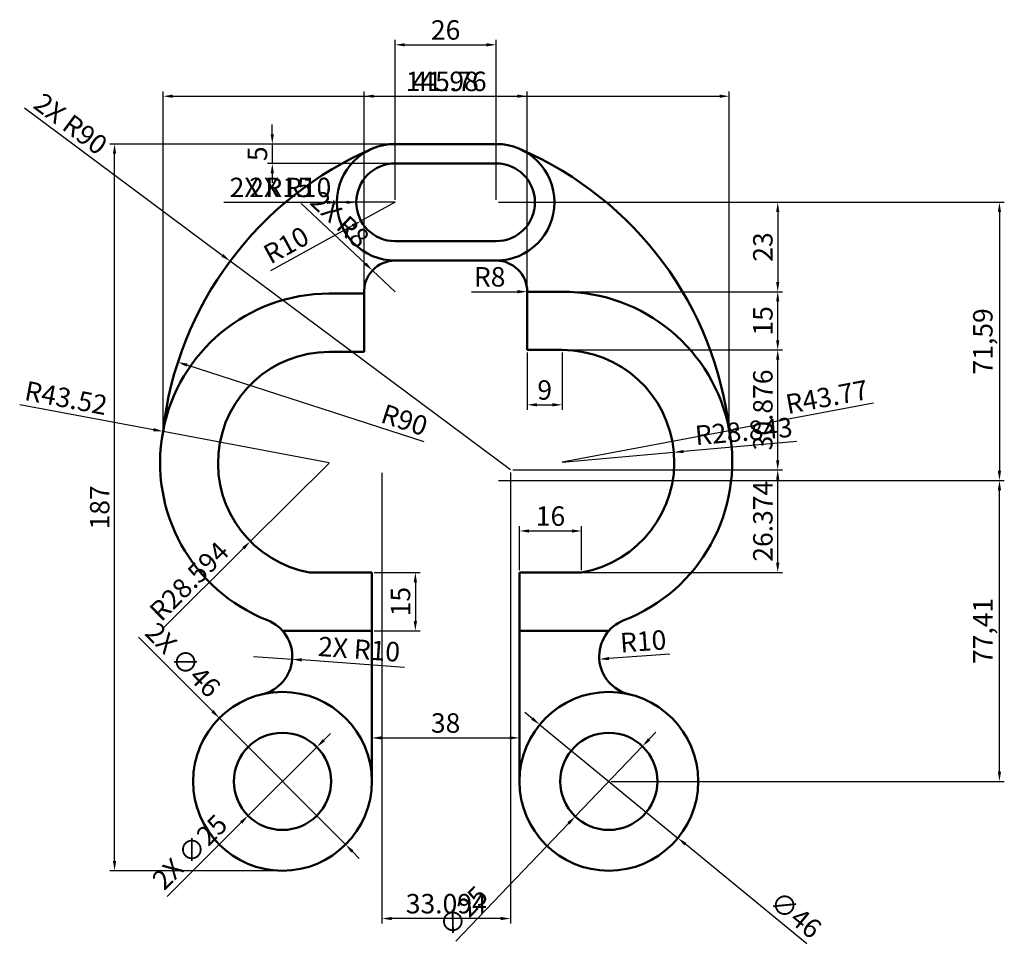
# Model space of a CAD drawing. Units: millimetres. Extents: x 2764 to 3018, y 1811 to 2049.
import ezdxf

# ---------------------------------------------------------------- set-up
doc = ezdxf.new("R2010")
doc.units = ezdxf.units.MM
doc.layers.add('M-DIMS', color=2, linetype='Continuous', lineweight=25)
doc.layers.add('M-OUTL', color=7, linetype='Continuous', lineweight=50)
doc.styles.get("Standard").update_dxf_attribs({"font": 'arial.ttf'})
doc.dimstyles.new('ISO-25', dxfattribs={"dimtxt": 5, "dimasz": 2.5, "dimexe": 1.25, "dimexo": 0.625, "dimtad": 1, "dimtxsty": 'Standard', "dimcen": 2.5, "dimadec": 0, "dimazin": 0, "dimtfac": 1, "dimtmove": 0, "dimatfit": 3, "dimfxl": 1, "dimarcsym": 0})

# ---------------------------------------------------------------- blocks, each defined once
blk = doc.blocks.new('*D1')
at = {"layer": 'Defpoints', "color": 0, "transparency": 16777216}
for p in [(2915.74, 1930.13), (3016.29, 1930.13), (2915.74, 1852.71)]:
    blk.add_point(p, dxfattribs=at)
at = {"layer": 'M-DIMS', "color": 0, "lineweight": -2, "transparency": 16777216}
for p, q in [((2916.37, 1930.13), (3017.54, 1930.13)), ((3016.29, 1855.21), (3016.29, 1927.63)), ((2916.37, 1852.71), (3017.54, 1852.71))]:
    blk.add_line(p, q, dxfattribs=at)
at = {"layer": 'M-DIMS', "color": 0, "transparency": 16777216}
for points in [[(3015.87, 1927.63), (3016.71, 1927.63), (3016.29, 1930.13)], [(3015.87, 1855.21), (3016.71, 1855.21), (3016.29, 1852.71)]]:
    blk.add_solid(points, dxfattribs=at)
at = {"layer": 'M-DIMS', "color": 0, "transparency": 16777216, "insert": (3012.66, 1891.42), "char_height": 5, "attachment_point": 5, "rotation": 90}
blk.add_mtext('77,41', dxfattribs=at)
blk = doc.blocks.new('*D2')
at = {"layer": 'Defpoints', "color": 0, "transparency": 16777216}
for p in [(2886.74, 2001.71), (2886.74, 1930.13), (3016.29, 1930.13)]:
    blk.add_point(p, dxfattribs=at)
at = {"layer": 'M-DIMS', "color": 0, "lineweight": -2, "transparency": 16777216}
for p, q in [((2887.37, 2001.71), (3017.54, 2001.71)), ((3016.29, 1999.21), (3016.29, 1932.63)), ((2887.37, 1930.13), (3017.54, 1930.13))]:
    blk.add_line(p, q, dxfattribs=at)
at = {"layer": 'M-DIMS', "color": 0, "transparency": 16777216}
for points in [[(3015.87, 1999.21), (3016.71, 1999.21), (3016.29, 2001.71)], [(3015.87, 1932.63), (3016.71, 1932.63), (3016.29, 1930.13)]]:
    blk.add_solid(points, dxfattribs=at)
at = {"layer": 'M-DIMS', "color": 0, "transparency": 16777216, "insert": (3012.66, 1965.92), "char_height": 5, "attachment_point": 5, "rotation": 90}
blk.add_mtext('71,59', dxfattribs=at)
blk = doc.blocks.new('*D3')
at = {"layer": 'Defpoints', "color": 0, "transparency": 16777216}
for p in [(2886.74, 2042.24), (2860.74, 2001.71), (2886.74, 2001.71)]:
    blk.add_point(p, dxfattribs=at)
at = {"layer": 'M-DIMS', "color": 0, "lineweight": -2, "transparency": 16777216}
for p, q in [((2860.74, 2002.34), (2860.74, 2043.49)), ((2886.74, 2002.34), (2886.74, 2043.49)), ((2863.24, 2042.24), (2884.24, 2042.24))]:
    blk.add_line(p, q, dxfattribs=at)
at = {"layer": 'M-DIMS', "color": 0, "transparency": 16777216}
for points in [[(2863.24, 2042.66), (2863.24, 2041.83), (2860.74, 2042.24)], [(2884.24, 2042.66), (2884.24, 2041.83), (2886.74, 2042.24)]]:
    blk.add_solid(points, dxfattribs=at)
at = {"layer": 'M-DIMS', "color": 0, "transparency": 16777216, "insert": (2873.74, 2045.42), "char_height": 5, "attachment_point": 5}
blk.add_mtext('26', dxfattribs=at)
blk = doc.blocks.new('*D4')
at = {"layer": 'Defpoints', "color": 0, "transparency": 16777216}
for p in [(2873.74, 2016.71), (2829.13, 2011.71), (2873.74, 2011.71)]:
    blk.add_point(p, dxfattribs=at)
at = {"layer": 'M-DIMS', "color": 0, "lineweight": -2, "transparency": 16777216}
for p, q in [((2829.13, 2019.21), (2829.13, 2021.71)), ((2873.12, 2016.71), (2827.88, 2016.71)), ((2829.13, 2016.71), (2829.13, 2011.71)), ((2873.12, 2011.71), (2827.88, 2011.71)), ((2829.13, 2009.21), (2829.13, 2006.71))]:
    blk.add_line(p, q, dxfattribs=at)
at = {"layer": 'M-DIMS', "color": 0, "transparency": 16777216}
for points in [[(2828.71, 2019.21), (2829.54, 2019.21), (2829.13, 2016.71)], [(2828.71, 2009.21), (2829.54, 2009.21), (2829.13, 2011.71)]]:
    blk.add_solid(points, dxfattribs=at)
at = {"layer": 'M-DIMS', "color": 0, "transparency": 16777216, "insert": (2825.96, 2014.21), "char_height": 5, "attachment_point": 5, "rotation": 90}
blk.add_mtext('5', dxfattribs=at)
blk = doc.blocks.new('*D5')
at = {"layer": 'Defpoints', "color": 0, "transparency": 16777216}
for p in [(2908.74, 1917.14), (2892.74, 1906.46), (2908.74, 1906.46)]:
    blk.add_point(p, dxfattribs=at)
at = {"layer": 'M-DIMS', "color": 0, "lineweight": -2, "transparency": 16777216}
for p, q in [((2892.74, 1907.09), (2892.74, 1918.39)), ((2895.24, 1917.14), (2906.24, 1917.14)), ((2908.74, 1907.09), (2908.74, 1918.39))]:
    blk.add_line(p, q, dxfattribs=at)
at = {"layer": 'M-DIMS', "color": 0, "transparency": 16777216}
for points in [[(2895.24, 1917.56), (2895.24, 1916.72), (2892.74, 1917.14)], [(2906.24, 1917.56), (2906.24, 1916.72), (2908.74, 1917.14)]]:
    blk.add_solid(points, dxfattribs=at)
at = {"layer": 'M-DIMS', "color": 0, "transparency": 16777216, "insert": (2900.74, 1920.32), "char_height": 5, "attachment_point": 5}
blk.add_mtext('16', dxfattribs=at)
blk = doc.blocks.new('*D6')
at = {"layer": 'Defpoints', "color": 0, "transparency": 16777216}
for p in [(2894.74, 1963.71), (2903.74, 1963.71), (2903.74, 1949.6)]:
    blk.add_point(p, dxfattribs=at)
at = {"layer": 'M-DIMS', "color": 0, "lineweight": -2, "transparency": 16777216}
for p, q in [((2894.74, 1963.09), (2894.74, 1948.35)), ((2903.74, 1963.09), (2903.74, 1948.35)), ((2897.24, 1949.6), (2901.24, 1949.6))]:
    blk.add_line(p, q, dxfattribs=at)
at = {"layer": 'M-DIMS', "color": 0, "transparency": 16777216}
for points in [[(2897.24, 1950.02), (2897.24, 1949.19), (2894.74, 1949.6)], [(2901.24, 1950.02), (2901.24, 1949.19), (2903.74, 1949.6)]]:
    blk.add_solid(points, dxfattribs=at)
at = {"layer": 'M-DIMS', "color": 0, "transparency": 16777216, "insert": (2899.24, 1952.78), "char_height": 5, "attachment_point": 5}
blk.add_mtext('9', dxfattribs=at)
blk = doc.blocks.new('*D7')
at = {"layer": 'Defpoints', "color": 0, "transparency": 16777216}
for p in [(2854.74, 1906.46), (2854.74, 1891.46), (2865.95, 1891.46)]:
    blk.add_point(p, dxfattribs=at)
at = {"layer": 'M-DIMS', "color": 0, "lineweight": -2, "transparency": 16777216}
for p, q in [((2855.37, 1906.46), (2867.2, 1906.46)), ((2865.95, 1903.96), (2865.95, 1893.96)), ((2855.37, 1891.46), (2867.2, 1891.46))]:
    blk.add_line(p, q, dxfattribs=at)
at = {"layer": 'M-DIMS', "color": 0, "transparency": 16777216}
for points in [[(2865.54, 1903.96), (2866.37, 1903.96), (2865.95, 1906.46)], [(2865.54, 1893.96), (2866.37, 1893.96), (2865.95, 1891.46)]]:
    blk.add_solid(points, dxfattribs=at)
at = {"layer": 'M-DIMS', "color": 0, "transparency": 16777216, "insert": (2862.78, 1898.96), "char_height": 5, "attachment_point": 5, "rotation": 90}
blk.add_mtext('15', dxfattribs=at)
blk = doc.blocks.new('*D8')
at = {"layer": 'Defpoints', "color": 0, "transparency": 16777216}
for p in [(2892.74, 1863.9), (2854.74, 1852.71), (2892.74, 1852.71)]:
    blk.add_point(p, dxfattribs=at)
at = {"layer": 'M-DIMS', "color": 0, "lineweight": -2, "transparency": 16777216}
for p, q in [((2854.74, 1853.34), (2854.74, 1865.15)), ((2857.24, 1863.9), (2890.24, 1863.9)), ((2892.74, 1853.34), (2892.74, 1865.15))]:
    blk.add_line(p, q, dxfattribs=at)
at = {"layer": 'M-DIMS', "color": 0, "transparency": 16777216}
for points in [[(2857.24, 1864.31), (2857.24, 1863.48), (2854.74, 1863.9)], [(2890.24, 1864.31), (2890.24, 1863.48), (2892.74, 1863.9)]]:
    blk.add_solid(points, dxfattribs=at)
at = {"layer": 'M-DIMS', "color": 0, "transparency": 16777216, "insert": (2873.74, 1867.08), "char_height": 5, "attachment_point": 5}
blk.add_mtext('38', dxfattribs=at)
blk = doc.blocks.new('*D9')
at = {"layer": 'Defpoints', "color": 0, "transparency": 16777216}
for p in [(2897.96, 1867.3), (2933.53, 1838.13)]:
    blk.add_point(p, dxfattribs=at)
at = {"layer": 'M-DIMS', "color": 0, "lineweight": -2, "transparency": 16777216}
for p, q in [((2896.03, 1868.88), (2894.09, 1870.47)), ((2897.96, 1867.3), (2933.53, 1838.13)), ((2966.71, 1810.93), (2935.46, 1836.55))]:
    blk.add_line(p, q, dxfattribs=at)
at = {"layer": 'M-DIMS', "color": 0, "transparency": 16777216}
for points in [[(2896.29, 1869.2), (2895.76, 1868.56), (2897.96, 1867.3)], [(2935.73, 1836.87), (2935.2, 1836.22), (2933.53, 1838.13)]]:
    blk.add_solid(points, dxfattribs=at)
at = {"layer": 'M-DIMS', "color": 0, "transparency": 16777216, "insert": (2963.46, 1817.88), "char_height": 5, "attachment_point": 5, "rotation": 320.6521}
blk.add_mtext('∅46', dxfattribs=at)
blk = doc.blocks.new('*D10')
at = {"layer": 'Defpoints', "color": 0, "transparency": 16777216}
for p in [(2924.4, 1861.74), (2907.09, 1843.69)]:
    blk.add_point(p, dxfattribs=at)
at = {"layer": 'M-DIMS', "color": 0, "lineweight": -2, "transparency": 16777216}
for p, q in [((2926.13, 1863.54), (2927.86, 1865.34)), ((2924.4, 1861.74), (2907.09, 1843.69)), ((2876.33, 1811.61), (2905.36, 1841.89))]:
    blk.add_line(p, q, dxfattribs=at)
at = {"layer": 'M-DIMS', "color": 0, "transparency": 16777216}
for points in [[(2925.83, 1863.83), (2926.43, 1863.25), (2924.4, 1861.74)], [(2905.06, 1842.18), (2905.66, 1841.6), (2907.09, 1843.69)]]:
    blk.add_solid(points, dxfattribs=at)
at = {"layer": 'M-DIMS', "color": 0, "transparency": 16777216, "insert": (2878.74, 1818.92), "char_height": 5, "attachment_point": 5, "rotation": 46.2}
blk.add_mtext('∅25', dxfattribs=at)
blk = doc.blocks.new('*D11')
at = {"layer": 'Defpoints', "color": 0, "transparency": 16777216}
for p in [(2804.83, 1960.59), (2890.45, 1932.84)]:
    blk.add_point(p, dxfattribs=at)
at = {"layer": 'M-DIMS', "color": 0, "lineweight": -2, "transparency": 16777216}
blk.add_line((2868.23, 1940.04), (2807.21, 1959.82), dxfattribs=at)
at = {"layer": 'M-DIMS', "color": 0, "transparency": 16777216}
blk.add_solid([(2807.34, 1960.21), (2807.08, 1959.42), (2804.83, 1960.59)], dxfattribs=at)
at = {"layer": 'M-DIMS', "color": 0, "transparency": 16777216, "insert": (2862.94, 1945.1), "char_height": 5, "attachment_point": 5, "rotation": 342.0412}
blk.add_mtext('R90', dxfattribs=at)
blk = doc.blocks.new('*D12')
at = {"layer": 'Defpoints', "color": 0, "transparency": 16777216}
for p in [(2886.74, 1978.71), (2894.74, 1978.71)]:
    blk.add_point(p, dxfattribs=at)
at = {"layer": 'M-DIMS', "color": 0, "lineweight": -2, "transparency": 16777216}
blk.add_line((2880.42, 1978.71), (2892.24, 1978.71), dxfattribs=at)
blk.add_arc((2886.74, 1978.71), 8, 351.0475, 355.5238, dxfattribs=at)
at = {"layer": 'M-DIMS', "color": 0, "transparency": 16777216}
blk.add_solid([(2892.24, 1979.13), (2892.24, 1978.3), (2894.74, 1978.71)], dxfattribs=at)
at = {"layer": 'M-DIMS', "color": 0, "transparency": 16777216, "insert": (2885.08, 1981.89), "char_height": 5, "attachment_point": 5}
blk.add_mtext('R8', dxfattribs=at)
blk = doc.blocks.new('*D13')
at = {"layer": 'Defpoints', "color": 0, "transparency": 16777216}
for p in [(2913.29, 1884.14), (2923.26, 1884.85)]:
    blk.add_point(p, dxfattribs=at)
at = {"layer": 'M-DIMS', "color": 0, "lineweight": -2, "transparency": 16777216}
blk.add_line((2931.42, 1885.42), (2915.78, 1884.31), dxfattribs=at)
at = {"layer": 'M-DIMS', "color": 0, "transparency": 16777216}
blk.add_solid([(2915.75, 1884.73), (2915.81, 1883.9), (2913.29, 1884.14)], dxfattribs=at)
at = {"layer": 'M-DIMS', "color": 0, "transparency": 16777216, "insert": (2924.63, 1888.13), "char_height": 5, "attachment_point": 5, "rotation": 4.0574}
blk.add_mtext('R10', dxfattribs=at)
blk = doc.blocks.new('*D14')
at = {"layer": 'Defpoints', "color": 0, "transparency": 16777216}
for p in [(2860.74, 2001.71), (2851.97, 1996.91)]:
    blk.add_point(p, dxfattribs=at)
at = {"layer": 'M-DIMS', "color": 0, "lineweight": -2, "transparency": 16777216}
for p, q in [((2860.74, 2001.71), (2851.97, 1996.91)), ((2828.75, 1984.2), (2849.78, 1995.71))]:
    blk.add_line(p, q, dxfattribs=at)
at = {"layer": 'M-DIMS', "color": 0, "transparency": 16777216}
blk.add_solid([(2849.58, 1996.08), (2849.98, 1995.35), (2851.97, 1996.91)], dxfattribs=at)
at = {"layer": 'M-DIMS', "color": 0, "transparency": 16777216, "insert": (2833, 1990.15), "char_height": 5, "attachment_point": 5, "rotation": 28.6971}
blk.add_mtext('R10', dxfattribs=at)
blk = doc.blocks.new('*D15')
at = {"layer": 'Defpoints', "color": 0, "transparency": 16777216}
for p in [(2946.76, 2029.01), (2801, 1942.76), (2946.76, 1943.03)]:
    blk.add_point(p, dxfattribs=at)
at = {"layer": 'M-DIMS', "color": 0, "lineweight": -2, "transparency": 16777216}
for p, q in [((2801, 1943.39), (2801, 2030.26)), ((2946.76, 1943.65), (2946.76, 2030.26)), ((2803.5, 2029.01), (2944.26, 2029.01))]:
    blk.add_line(p, q, dxfattribs=at)
at = {"layer": 'M-DIMS', "color": 0, "transparency": 16777216}
for points in [[(2803.5, 2029.43), (2803.5, 2028.6), (2801, 2029.01)], [(2944.26, 2029.43), (2944.26, 2028.6), (2946.76, 2029.01)]]:
    blk.add_solid(points, dxfattribs=at)
at = {"layer": 'M-DIMS', "color": 0, "transparency": 16777216, "insert": (2873.88, 2032.19), "char_height": 5, "attachment_point": 5}
blk.add_mtext('145.76', dxfattribs=at)
blk = doc.blocks.new('*D16')
at = {"layer": 'Defpoints', "color": 0, "transparency": 16777216}
for p in [(2788.52, 2016.71), (2860.74, 2016.71), (2831.74, 1829.71)]:
    blk.add_point(p, dxfattribs=at)
at = {"layer": 'M-DIMS', "color": 0, "lineweight": -2, "transparency": 16777216}
for p, q in [((2860.12, 2016.71), (2787.27, 2016.71)), ((2788.52, 1832.21), (2788.52, 2014.21)), ((2831.12, 1829.71), (2787.27, 1829.71))]:
    blk.add_line(p, q, dxfattribs=at)
at = {"layer": 'M-DIMS', "color": 0, "transparency": 16777216}
for points in [[(2788.11, 2014.21), (2788.94, 2014.21), (2788.52, 2016.71)], [(2788.11, 1832.21), (2788.94, 1832.21), (2788.52, 1829.71)]]:
    blk.add_solid(points, dxfattribs=at)
at = {"layer": 'M-DIMS', "color": 0, "transparency": 16777216, "insert": (2785.35, 1923.21), "char_height": 5, "attachment_point": 5, "rotation": 90}
blk.add_mtext('187', dxfattribs=at)
blk = doc.blocks.new('*D17')
at = {"layer": 'Defpoints', "color": 0, "transparency": 16777216}
for p in [(2894.74, 2029.01), (2852.76, 1963.21), (2894.74, 1963.71)]:
    blk.add_point(p, dxfattribs=at)
at = {"layer": 'M-DIMS', "color": 0, "lineweight": -2, "transparency": 16777216}
for p, q in [((2852.76, 1963.83), (2852.76, 2030.26)), ((2894.74, 1964.34), (2894.74, 2030.26)), ((2855.26, 2029.01), (2892.24, 2029.01))]:
    blk.add_line(p, q, dxfattribs=at)
at = {"layer": 'M-DIMS', "color": 0, "transparency": 16777216}
for points in [[(2855.26, 2029.43), (2855.26, 2028.6), (2852.76, 2029.01)], [(2892.24, 2029.43), (2892.24, 2028.6), (2894.74, 2029.01)]]:
    blk.add_solid(points, dxfattribs=at)
at = {"layer": 'M-DIMS', "color": 0, "transparency": 16777216, "insert": (2873.75, 2032.19), "char_height": 5, "attachment_point": 5}
blk.add_mtext('41.98', dxfattribs=at)
blk = doc.blocks.new('*D18')
at = {"layer": 'Defpoints', "color": 0, "transparency": 16777216}
for p in [(2894.74, 1978.71), (2959.22, 1978.71), (2894.74, 1963.71)]:
    blk.add_point(p, dxfattribs=at)
at = {"layer": 'M-DIMS', "color": 0, "lineweight": -2, "transparency": 16777216}
for p, q in [((2895.37, 1978.71), (2960.47, 1978.71)), ((2959.22, 1966.21), (2959.22, 1976.21)), ((2895.37, 1963.71), (2960.47, 1963.71))]:
    blk.add_line(p, q, dxfattribs=at)
at = {"layer": 'M-DIMS', "color": 0, "transparency": 16777216}
for points in [[(2958.8, 1976.21), (2959.64, 1976.21), (2959.22, 1978.71)], [(2958.8, 1966.21), (2959.64, 1966.21), (2959.22, 1963.71)]]:
    blk.add_solid(points, dxfattribs=at)
at = {"layer": 'M-DIMS', "color": 0, "transparency": 16777216, "insert": (2956.04, 1971.21), "char_height": 5, "attachment_point": 5, "rotation": 90}
blk.add_mtext('15', dxfattribs=at)
blk = doc.blocks.new('*D19')
at = {"layer": 'Defpoints', "color": 0, "transparency": 16777216}
for p in [(2886.74, 2001.71), (2894.74, 1978.71), (2959.22, 1978.71)]:
    blk.add_point(p, dxfattribs=at)
at = {"layer": 'M-DIMS', "color": 0, "lineweight": -2, "transparency": 16777216}
for p, q in [((2887.37, 2001.71), (2960.47, 2001.71)), ((2959.22, 1999.21), (2959.22, 1981.21)), ((2895.37, 1978.71), (2960.47, 1978.71))]:
    blk.add_line(p, q, dxfattribs=at)
at = {"layer": 'M-DIMS', "color": 0, "transparency": 16777216}
for points in [[(2958.8, 1999.21), (2959.64, 1999.21), (2959.22, 2001.71)], [(2958.8, 1981.21), (2959.64, 1981.21), (2959.22, 1978.71)]]:
    blk.add_solid(points, dxfattribs=at)
at = {"layer": 'M-DIMS', "color": 0, "transparency": 16777216, "insert": (2956.04, 1990.21), "char_height": 5, "attachment_point": 5, "rotation": 90}
blk.add_mtext('23', dxfattribs=at)
blk = doc.blocks.new('*D20')
at = {"layer": 'Defpoints', "color": 0, "transparency": 16777216}
for p in [(2890.45, 1932.84), (2959.22, 1932.84), (2908.74, 1906.46)]:
    blk.add_point(p, dxfattribs=at)
at = {"layer": 'M-DIMS', "color": 0, "lineweight": -2, "transparency": 16777216}
for p, q in [((2891.07, 1932.84), (2960.47, 1932.84)), ((2959.22, 1908.96), (2959.22, 1930.34)), ((2909.37, 1906.46), (2960.47, 1906.46))]:
    blk.add_line(p, q, dxfattribs=at)
at = {"layer": 'M-DIMS', "color": 0, "transparency": 16777216}
for points in [[(2958.8, 1930.34), (2959.64, 1930.34), (2959.22, 1932.84)], [(2958.8, 1908.96), (2959.64, 1908.96), (2959.22, 1906.46)]]:
    blk.add_solid(points, dxfattribs=at)
at = {"layer": 'M-DIMS', "color": 0, "transparency": 16777216, "insert": (2956.04, 1919.65), "char_height": 5, "attachment_point": 5, "rotation": 90}
blk.add_mtext('26.374', dxfattribs=at)
blk = doc.blocks.new('*D21')
at = {"layer": 'Defpoints', "color": 0, "transparency": 16777216}
for p in [(2894.74, 1963.71), (2959.22, 1963.71), (2890.45, 1932.84)]:
    blk.add_point(p, dxfattribs=at)
at = {"layer": 'M-DIMS', "color": 0, "lineweight": -2, "transparency": 16777216}
for p, q in [((2895.37, 1963.71), (2960.47, 1963.71)), ((2959.22, 1935.34), (2959.22, 1961.21)), ((2891.07, 1932.84), (2960.47, 1932.84))]:
    blk.add_line(p, q, dxfattribs=at)
at = {"layer": 'M-DIMS', "color": 0, "transparency": 16777216}
for points in [[(2958.8, 1961.21), (2959.64, 1961.21), (2959.22, 1963.71)], [(2958.8, 1935.34), (2959.64, 1935.34), (2959.22, 1932.84)]]:
    blk.add_solid(points, dxfattribs=at)
at = {"layer": 'M-DIMS', "color": 0, "transparency": 16777216, "insert": (2956.04, 1948.28), "char_height": 5, "attachment_point": 5, "rotation": 90}
blk.add_mtext('30.876', dxfattribs=at)
blk = doc.blocks.new('*D22')
at = {"layer": 'Defpoints', "color": 0, "transparency": 16777216}
for p in [(2857.35, 1932.7), (2890.45, 1932.84), (2857.35, 1817.41)]:
    blk.add_point(p, dxfattribs=at)
at = {"layer": 'M-DIMS', "color": 0, "lineweight": -2, "transparency": 16777216}
for p, q in [((2857.35, 1932.08), (2857.35, 1816.16)), ((2890.45, 1932.21), (2890.45, 1816.16)), ((2887.95, 1817.41), (2859.85, 1817.41))]:
    blk.add_line(p, q, dxfattribs=at)
at = {"layer": 'M-DIMS', "color": 0, "transparency": 16777216}
for points in [[(2859.85, 1817.83), (2859.85, 1817), (2857.35, 1817.41)], [(2887.95, 1817.83), (2887.95, 1817), (2890.45, 1817.41)]]:
    blk.add_solid(points, dxfattribs=at)
at = {"layer": 'M-DIMS', "color": 0, "transparency": 16777216, "insert": (2873.9, 1820.59), "char_height": 5, "attachment_point": 5}
blk.add_mtext('33.094', dxfattribs=at)
blk = doc.blocks.new('*D23')
at = {"layer": 'Defpoints', "color": 0, "transparency": 16777216}
for p in [(2818.26, 1986.59), (2890.45, 1932.84)]:
    blk.add_point(p, dxfattribs=at)
at = {"layer": 'M-DIMS', "color": 0, "lineweight": -2, "transparency": 16777216}
for p, q in [((2765.32, 2026.01), (2816.26, 1988.08)), ((2890.45, 1932.84), (2818.26, 1986.59))]:
    blk.add_line(p, q, dxfattribs=at)
at = {"layer": 'M-DIMS', "color": 0, "transparency": 16777216}
blk.add_solid([(2816.5, 1988.41), (2816.01, 1987.75), (2818.26, 1986.59)], dxfattribs=at)
at = {"layer": 'M-DIMS', "color": 0, "transparency": 16777216, "insert": (2776.85, 2021.39), "char_height": 5, "attachment_point": 5, "rotation": 323.3297}
blk.add_mtext('2X R90', dxfattribs=at)
blk = doc.blocks.new('*D24')
at = {"layer": 'Defpoints', "color": 0, "transparency": 16777216}
for p in [(2801, 1942.76), (2843.76, 1934.69)]:
    blk.add_point(p, dxfattribs=at)
at = {"layer": 'M-DIMS', "color": 0, "lineweight": -2, "transparency": 16777216}
for p, q in [((2764.11, 1949.72), (2798.54, 1943.22)), ((2843.76, 1934.69), (2801, 1942.76))]:
    blk.add_line(p, q, dxfattribs=at)
at = {"layer": 'M-DIMS', "color": 0, "transparency": 16777216}
blk.add_solid([(2798.62, 1943.63), (2798.46, 1942.81), (2801, 1942.76)], dxfattribs=at)
at = {"layer": 'M-DIMS', "color": 0, "transparency": 16777216, "insert": (2775.93, 1950.73), "char_height": 5, "attachment_point": 5, "rotation": 349.3147}
blk.add_mtext('R43.52', dxfattribs=at)
blk = doc.blocks.new('*D25')
at = {"layer": 'Defpoints', "color": 0, "transparency": 16777216}
for p in [(2946.76, 1943.03), (2903.74, 1934.95)]:
    blk.add_point(p, dxfattribs=at)
at = {"layer": 'M-DIMS', "color": 0, "lineweight": -2, "transparency": 16777216}
for p, q in [((2983.83, 1949.99), (2949.22, 1943.49)), ((2903.74, 1934.95), (2946.76, 1943.03))]:
    blk.add_line(p, q, dxfattribs=at)
at = {"layer": 'M-DIMS', "color": 0, "transparency": 16777216}
blk.add_solid([(2949.14, 1943.9), (2949.29, 1943.08), (2946.76, 1943.03)], dxfattribs=at)
at = {"layer": 'M-DIMS', "color": 0, "transparency": 16777216, "insert": (2971.98, 1951), "char_height": 5, "attachment_point": 5, "rotation": 10.6432}
blk.add_mtext('R43.77', dxfattribs=at)
blk = doc.blocks.new('*D26')
at = {"layer": 'Defpoints', "color": 0, "transparency": 16777216}
for p in [(2843.76, 1934.61), (2823.47, 1914.47)]:
    blk.add_point(p, dxfattribs=at)
at = {"layer": 'M-DIMS', "color": 0, "lineweight": -2, "transparency": 16777216}
for p, q in [((2843.76, 1934.61), (2823.47, 1914.47)), ((2800.92, 1892.08), (2821.69, 1912.71))]:
    blk.add_line(p, q, dxfattribs=at)
at = {"layer": 'M-DIMS', "color": 0, "transparency": 16777216}
blk.add_solid([(2821.4, 1913), (2821.99, 1912.41), (2823.47, 1914.47)], dxfattribs=at)
at = {"layer": 'M-DIMS', "color": 0, "transparency": 16777216, "insert": (2808.18, 1903.77), "char_height": 5, "attachment_point": 5, "rotation": 44.7927}
blk.add_mtext('R28.594', dxfattribs=at)
blk = doc.blocks.new('*D27')
at = {"layer": 'Defpoints', "color": 0, "transparency": 16777216}
for p in [(2932.48, 1937.38), (2903.74, 1934.87)]:
    blk.add_point(p, dxfattribs=at)
at = {"layer": 'M-DIMS', "color": 0, "lineweight": -2, "transparency": 16777216}
for p, q in [((2964.15, 1940.15), (2934.97, 1937.6)), ((2903.74, 1934.87), (2932.48, 1937.38))]:
    blk.add_line(p, q, dxfattribs=at)
at = {"layer": 'M-DIMS', "color": 0, "transparency": 16777216}
blk.add_solid([(2934.93, 1938.01), (2935.01, 1937.18), (2932.48, 1937.38)], dxfattribs=at)
at = {"layer": 'M-DIMS', "color": 0, "transparency": 16777216, "insert": (2950.53, 1942.15), "char_height": 5, "attachment_point": 5, "rotation": 4.9917}
blk.add_mtext('R28.843', dxfattribs=at)
blk = doc.blocks.new('*D28')
at = {"layer": 'Defpoints', "color": 0, "transparency": 16777216}
for p in [(2815.5, 1869), (2847.99, 1836.43)]:
    blk.add_point(p, dxfattribs=at)
at = {"layer": 'M-DIMS', "color": 0, "lineweight": -2, "transparency": 16777216}
for p, q in [((2794.73, 1889.82), (2813.74, 1870.77)), ((2847.99, 1836.43), (2815.5, 1869)), ((2849.75, 1834.66), (2851.52, 1832.89))]:
    blk.add_line(p, q, dxfattribs=at)
at = {"layer": 'M-DIMS', "color": 0, "transparency": 16777216}
for points in [[(2814.03, 1871.06), (2813.44, 1870.47), (2815.5, 1869)], [(2850.05, 1834.95), (2849.46, 1834.37), (2847.99, 1836.43)]]:
    blk.add_solid(points, dxfattribs=at)
at = {"layer": 'M-DIMS', "color": 0, "transparency": 16777216, "insert": (2805.7, 1883.52), "char_height": 5, "attachment_point": 5, "rotation": 314.9266}
blk.add_mtext('2X ∅46', dxfattribs=at)
blk = doc.blocks.new('*D29')
at = {"layer": 'Defpoints', "color": 0, "transparency": 16777216}
for p in [(2840.6, 1861.54), (2822.89, 1843.89)]:
    blk.add_point(p, dxfattribs=at)
at = {"layer": 'M-DIMS', "color": 0, "lineweight": -2, "transparency": 16777216}
for p, q in [((2842.37, 1863.3), (2844.14, 1865.07)), ((2840.6, 1861.54), (2822.89, 1843.89)), ((2802.03, 1823.1), (2821.12, 1842.13))]:
    blk.add_line(p, q, dxfattribs=at)
at = {"layer": 'M-DIMS', "color": 0, "transparency": 16777216}
for points in [[(2842.08, 1863.6), (2842.66, 1863.01), (2840.6, 1861.54)], [(2820.83, 1842.42), (2821.41, 1841.83), (2822.89, 1843.89)]]:
    blk.add_solid(points, dxfattribs=at)
at = {"layer": 'M-DIMS', "color": 0, "transparency": 16777216, "insert": (2808.35, 1834.08), "char_height": 5, "attachment_point": 5, "rotation": 44.899}
blk.add_mtext('2X ∅25', dxfattribs=at)
blk = doc.blocks.new('*D30')
at = {"layer": 'Defpoints', "color": 0, "transparency": 16777216}
for p in [(2845.74, 2001.71), (2860.74, 2001.71)]:
    blk.add_point(p, dxfattribs=at)
at = {"layer": 'M-DIMS', "color": 0, "lineweight": -2, "transparency": 16777216}
for p, q in [((2816.68, 2001.71), (2843.24, 2001.71)), ((2860.74, 2001.71), (2845.74, 2001.71))]:
    blk.add_line(p, q, dxfattribs=at)
at = {"layer": 'M-DIMS', "color": 0, "transparency": 16777216}
blk.add_solid([(2843.24, 2002.13), (2843.24, 2001.3), (2845.74, 2001.71)], dxfattribs=at)
at = {"layer": 'M-DIMS', "color": 0, "transparency": 16777216, "insert": (2828.71, 2004.89), "char_height": 5, "attachment_point": 5, "rotation": 359.9984}
blk.add_mtext('2X R15', dxfattribs=at)
blk = doc.blocks.new('*D31')
at = {"layer": 'Defpoints', "color": 0, "transparency": 16777216}
for p in [(2850.74, 2001.71), (2860.74, 2001.71)]:
    blk.add_point(p, dxfattribs=at)
at = {"layer": 'M-DIMS', "color": 0, "lineweight": -2, "transparency": 16777216}
for p, q in [((2821.74, 2001.72), (2848.24, 2001.71)), ((2860.74, 2001.71), (2850.74, 2001.71))]:
    blk.add_line(p, q, dxfattribs=at)
at = {"layer": 'M-DIMS', "color": 0, "transparency": 16777216}
blk.add_solid([(2848.24, 2002.13), (2848.24, 2001.3), (2850.74, 2001.71)], dxfattribs=at)
at = {"layer": 'M-DIMS', "color": 0, "transparency": 16777216, "insert": (2833.74, 2004.89), "char_height": 5, "attachment_point": 5, "rotation": 359.9977}
blk.add_mtext('2X R10', dxfattribs=at)
blk = doc.blocks.new('*D32')
at = {"layer": 'Defpoints', "color": 0, "transparency": 16777216}
for p in [(2824.26, 1884.85), (2834.23, 1884.13)]:
    blk.add_point(p, dxfattribs=at)
at = {"layer": 'M-DIMS', "color": 0, "lineweight": -2, "transparency": 16777216}
for p, q in [((2824.26, 1884.85), (2834.23, 1884.13)), ((2863.17, 1882.04), (2836.73, 1883.95))]:
    blk.add_line(p, q, dxfattribs=at)
at = {"layer": 'M-DIMS', "color": 0, "transparency": 16777216}
blk.add_solid([(2836.76, 1884.37), (2836.7, 1883.54), (2834.23, 1884.13)], dxfattribs=at)
at = {"layer": 'M-DIMS', "color": 0, "transparency": 16777216, "insert": (2851.42, 1886.08), "char_height": 5, "attachment_point": 5, "rotation": 355.8695}
blk.add_mtext('2X R10', dxfattribs=at)
blk = doc.blocks.new('*D33')
at = {"layer": 'Defpoints', "color": 0, "transparency": 16777216}
for p in [(2854.91, 1984.19), (2860.74, 1978.71)]:
    blk.add_point(p, dxfattribs=at)
at = {"layer": 'M-DIMS', "color": 0, "lineweight": -2, "transparency": 16777216}
for p, q in [((2836.57, 2001.4), (2853.09, 1985.9)), ((2860.74, 1978.71), (2854.91, 1984.19))]:
    blk.add_line(p, q, dxfattribs=at)
at = {"layer": 'M-DIMS', "color": 0, "transparency": 16777216}
blk.add_solid([(2853.37, 1986.2), (2852.8, 1985.6), (2854.91, 1984.19)], dxfattribs=at)
at = {"layer": 'M-DIMS', "color": 0, "transparency": 16777216, "insert": (2846.1, 1996.82), "char_height": 5, "attachment_point": 5, "rotation": 316.8098}
blk.add_mtext('2X R8', dxfattribs=at)

msp = doc.modelspace()

# ---------------------------------------------------------------- linework, layer by layer
at = {"layer": 'M-OUTL'}
for p, q in [((2860.7447, 2016.7136), (2886.7447, 2016.7136)), ((2860.7447, 2011.7136), (2886.7447, 2011.7136)), ((2860.7447, 1991.7136), (2886.7447, 1991.7136)), ((2860.7447, 1986.7136), (2886.7447, 1986.7136)), ((2852.7607, 1978.2089), (2843.7607, 1978.2089)), ((2852.7607, 1978.2089), (2852.7607, 1963.2089)), ((2894.7447, 1978.7136), (2903.7447, 1978.7136)), ((2894.7447, 1978.7136), (2894.7447, 1963.7136)), ((2852.7607, 1963.2089), (2843.7607, 1963.2089)), ((2894.7447, 1963.7136), (2903.7447, 1963.7136)), ((2854.7447, 1906.4636), (2838.7447, 1906.4636)), ((2854.7447, 1852.7136), (2854.7447, 1906.4636)), ((2892.7447, 1906.4636), (2908.7447, 1906.4636)), ((2892.7447, 1852.7136), (2892.7447, 1906.4636)), ((2854.7447, 1891.4636), (2831.7624, 1891.4636)), ((2892.7447, 1891.4636), (2915.7679, 1891.4636))]:
    msp.add_line(p, q, dxfattribs=at)
for centre, radius in [((2831.7447, 1852.7136), 23), ((2915.7447, 1852.7136), 23), ((2831.7447, 1852.7136), 12.5), ((2915.7447, 1852.7136), 12.5)]:
    msp.add_circle(centre, radius, dxfattribs=at)
for centre, radius, start, end in [((2890.4489, 1932.838), 90, 112.989284, 173.670531), ((2860.7447, 2001.7136), 15, 90, 270), ((2886.7447, 2001.7136), 15, 270, 90), ((2857.3546, 1932.701), 90, 6.589579, 66.548893), ((2860.7447, 2001.7136), 10, 90, 270), ((2886.7447, 2001.7136), 10, 270, 90), ((2860.7447, 1978.7136), 8, 90, 183.61669), ((2886.7447, 1978.7136), 8, 0, 90), ((2843.7607, 1934.6912), 43.5177, 90, 248.62932), ((2903.7447, 1934.9453), 43.7683, 291.286757, 90), ((2843.7607, 1934.6146), 28.5944, 90, 259.897084), ((2903.7447, 1934.8703), 28.8433, 279.982667, 90), ((2824.2588, 1884.8533), 10, 283.111476, 68.62932), ((2923.2645, 1884.8454), 10, 111.286757, 256.82812)]:
    msp.add_arc(centre, radius, start, end, dxfattribs=at)

# ---------------------------------------------------------------- dimensions: what is measured, and where the dimension line sits
at = {"layer": 'M-DIMS'}
for base, p1, p2, override, picture, middle in [((2886.7447, 2042.2417), (2860.7447, 2001.7136), (2886.7447, 2001.7136), {"dimclrd": 0, "dimclre": 0, "dimclrt": 0}, '*D3', (2873.7447, 2045.4196)), ((2946.76, 2029.0136), (2800.9975, 1942.7601), (2946.76, 1943.0291), {"dimdec": 2, "dimlfac": 1, "dimrnd": 0, "dimzin": 0, "dimdsep": 46, "dimlunit": 2}, '*D15', (2873.8788, 2032.1915)), ((2894.7447, 2029.0136), (2852.7607, 1963.2089), (2894.7447, 1963.7136), {"dimdec": 2, "dimlfac": 1, "dimrnd": 0, "dimzin": 0, "dimdsep": 46, "dimlunit": 2}, '*D17', (2873.7527, 2032.1915)), ((2903.7447, 1949.6033), (2894.7447, 1963.7136), (2903.7447, 1963.7136), {"dimclrd": 0, "dimclre": 0, "dimclrt": 0}, '*D6', (2899.2447, 1952.7812)), ((2857.3546, 1817.4136), (2890.4489, 1932.838), (2857.3546, 1932.701), {"dimdec": 3, "dimlfac": 1, "dimrnd": 0, "dimzin": 0, "dimdsep": 46, "dimlunit": 2}, '*D22', (2873.9018, 1820.5932)), ((2908.7447, 1917.1406), (2892.7447, 1906.4636), (2908.7447, 1906.4636), {"dimclrd": 0, "dimclre": 0, "dimclrt": 0}, '*D5', (2900.7447, 1920.3184)), ((2892.7447, 1863.8968), (2854.7447, 1852.7136), (2892.7447, 1852.7136), {"dimclrd": 0, "dimclre": 0, "dimclrt": 0}, '*D8', (2873.7447, 1867.0764))]:
    dim = msp.add_linear_dim(base=base, p1=p1, p2=p2, dimstyle='ISO-25', override=override, dxfattribs=at)
    dim.commit()
    dim.dimension.update_dxf_attribs({"geometry": picture, "text_midpoint": middle})
dim = msp.add_radius_dim(center=(2890.4489, 1932.838), mpoint=(2818.2612, 1986.5868), text='2X <>', dimstyle='ISO-25', override={"dimdec": 0, "dimlfac": 1, "dimrnd": 0, "dimzin": 0, "dimdsep": 46, "dimlunit": 2}, dxfattribs=at)
dim.commit()
dim.dimension.update_dxf_attribs({"geometry": '*D23', "text_midpoint": (2774.9486, 2018.8361), "dimtype": 164})
for base, p1, p2, override, picture, middle in [((2829.1267, 2011.7136), (2873.7447, 2016.7136), (2873.7447, 2011.7136), {"dimclrd": 0, "dimclre": 0, "dimclrt": 0}, '*D4', (2825.9591, 2014.2136)), ((2788.525, 2016.7136), (2831.7447, 1829.7136), (2860.7447, 2016.7136), {"dimdec": 0, "dimlfac": 1, "dimrnd": 0, "dimzin": 0, "dimdsep": 46, "dimlunit": 2}, '*D16', (2785.3471, 1923.2136)), ((3016.2901, 1930.1268), (2886.7447, 2001.7136), (2886.7447, 1930.1268), {"dimclrd": 0, "dimclre": 0, "dimclrt": 0}, '*D2', (3012.6603, 1965.9202)), ((2959.221, 1978.7136), (2886.7447, 2001.7136), (2894.7447, 1978.7136), {"dimdec": 0, "dimlfac": 1, "dimrnd": 0, "dimzin": 0, "dimdsep": 46, "dimlunit": 2}, '*D19', (2956.0415, 1990.2136)), ((2959.221, 1978.7136), (2894.7447, 1963.7136), (2894.7447, 1978.7136), {"dimdec": 0, "dimlfac": 1, "dimrnd": 0, "dimzin": 0, "dimdsep": 46, "dimlunit": 2}, '*D18', (2956.0432, 1971.2136)), ((2959.221, 1963.7136), (2890.4489, 1932.838), (2894.7447, 1963.7136), {"dimdec": 3, "dimlfac": 1, "dimrnd": 0, "dimzin": 0, "dimdsep": 46, "dimlunit": 2}, '*D21', (2956.0415, 1948.2758)), ((2959.221, 1932.838), (2908.7447, 1906.4636), (2890.4489, 1932.838), {"dimdec": 3, "dimlfac": 1, "dimrnd": 0, "dimzin": 0, "dimdsep": 46, "dimlunit": 2}, '*D20', (2956.0415, 1919.6508)), ((3016.2901, 1930.1268), (2915.7447, 1852.7136), (2915.7447, 1930.1268), {"dimclrd": 0, "dimclre": 0, "dimclrt": 0}, '*D1', (3012.6603, 1891.4202)), ((2865.9529, 1891.4636), (2854.7447, 1906.4636), (2854.7447, 1891.4636), {"dimclrd": 0, "dimclre": 0, "dimclrt": 0}, '*D7', (2862.775, 1898.9636))]:
    dim = msp.add_linear_dim(base=base, p1=p1, p2=p2, angle=90, dimstyle='ISO-25', override=override, dxfattribs=at)
    dim.commit()
    dim.dimension.update_dxf_attribs({"geometry": picture, "text_midpoint": middle})
for center, mpoint, picture, middle in [((2860.7447, 2001.7136), (2845.7447, 2001.714), '*D30', (2828.7129, 2004.8923)), ((2860.7447, 2001.7136), (2850.7447, 2001.714), '*D31', (2833.7403, 2004.8926)), ((2860.7447, 1978.7136), (2854.912, 1984.189), '*D33', (2846.0954, 1996.8242)), ((2824.2588, 1884.8533), (2834.2328, 1884.133), '*D32', (2851.4222, 1886.0778))]:
    dim = msp.add_radius_dim(center=center, mpoint=mpoint, text='2X <>', dimstyle='ISO-25', override={"dimdec": 0, "dimlfac": 1, "dimrnd": 0, "dimzin": 0, "dimdsep": 46, "dimlunit": 2}, dxfattribs=at)
    dim.commit()
    dim.dimension.update_dxf_attribs({"geometry": picture, "text_midpoint": middle})
for center, mpoint, override, picture, middle in [((2860.7447, 2001.7136), (2851.973, 1996.9118), {"dimclrd": 0, "dimclre": 0, "dimclrt": 0}, '*D14', (2834.5272, 1987.3617)), ((2886.7447, 1978.7136), (2894.7447, 1978.7136), {"dimclrd": 0, "dimclre": 0, "dimclrt": 0}, '*D12', (2885.0832, 1978.7136)), ((2890.4489, 1932.838), (2804.8339, 1960.5879), {"dimclrd": 0, "dimclre": 0, "dimclrt": 0}, '*D11', (2861.956, 1942.0733)), ((2843.7607, 1934.6912), (2800.9975, 1942.7601), {"dimdec": 2, "dimlfac": 1, "dimrnd": 0, "dimzin": 0, "dimdsep": 46, "dimlunit": 2}, '*D24', (2775.3397, 1947.6014)), ((2903.7447, 1934.9453), (2946.76, 1943.029), {"dimdec": 2, "dimlfac": 1, "dimrnd": 0, "dimzin": 0, "dimdsep": 46, "dimlunit": 2}, '*D25', (2972.5692, 1947.8792)), ((2923.2645, 1884.8454), (2913.2896, 1884.1378), {"dimclrd": 0, "dimclre": 0, "dimclrt": 0}, '*D13', (2924.8508, 1884.9579))]:
    dim = msp.add_radius_dim(center=center, mpoint=mpoint, dimstyle='ISO-25', override=override, dxfattribs=at)
    dim.commit()
    dim.dimension.update_dxf_attribs({"geometry": picture, "text_midpoint": middle, "dimtype": 164})
for center, mpoint, picture, middle in [((2903.7447, 1934.8703), (2932.4787, 1937.38), '*D27', (2950.5284, 1942.1482)), ((2843.7607, 1934.6146), (2823.4684, 1914.4686), '*D26', (2808.1817, 1903.7701))]:
    dim = msp.add_radius_dim(center=center, mpoint=mpoint, dimstyle='ISO-25', override={"dimdec": 3, "dimlfac": 1, "dimrnd": 0, "dimzin": 0, "dimdsep": 46, "dimlunit": 2}, dxfattribs=at)
    dim.commit()
    dim.dimension.update_dxf_attribs({"geometry": picture, "text_midpoint": middle})
for p1, p2, picture, middle in [((2847.9873, 1836.4293), (2815.5021, 1868.9979), '*D28', (2803.3514, 1881.1798)), ((2840.5991, 1861.5368), (2822.8903, 1843.8904), '*D29', (2810.688, 1831.731))]:
    dim = msp.add_diameter_dim_2p(p1=p1, p2=p2, text='2X <>', dimstyle='ISO-25', override={"dimdec": 0, "dimlfac": 1, "dimrnd": 0, "dimzin": 0, "dimdsep": 46, "dimlunit": 2}, dxfattribs=at)
    dim.commit()
    dim.dimension.update_dxf_attribs({"geometry": picture, "text_midpoint": middle})
for p1, p2, picture, middle in [((2897.9586, 1867.2962), (2933.5309, 1838.131), '*D9', (2961.3538, 1815.3193)), ((2924.3965, 1861.7356), (2907.0929, 1843.6916), '*D10', (2881.138, 1816.6261))]:
    dim = msp.add_diameter_dim_2p(p1=p1, p2=p2, dimstyle='ISO-25', override={"dimclrd": 0, "dimclre": 0, "dimclrt": 0}, dxfattribs=at)
    dim.commit()
    dim.dimension.update_dxf_attribs({"geometry": picture, "text_midpoint": middle, "dimtype": 163})

doc.saveas('drawing.dxf')
